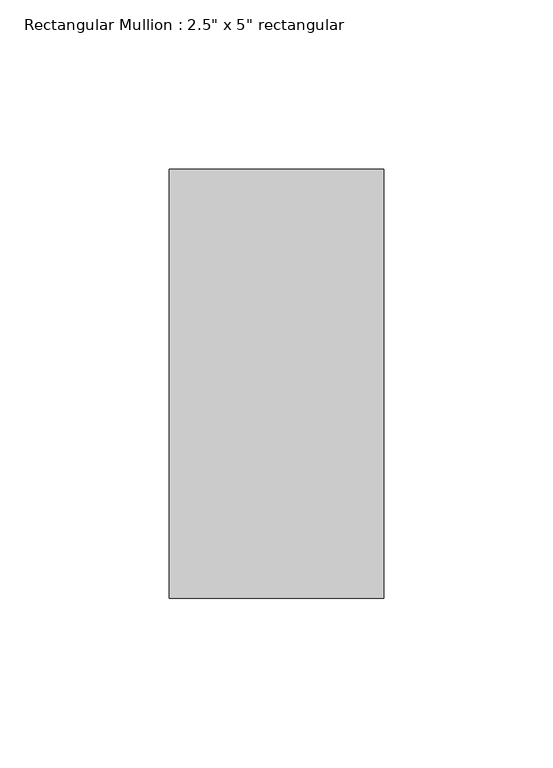
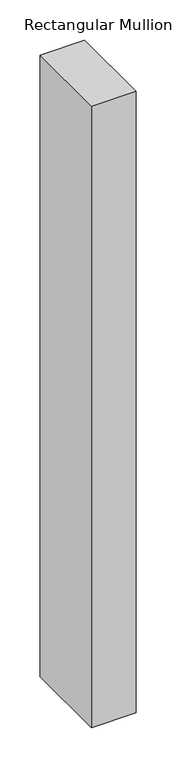
"""IFC4 building model written with IfcOpenShell, lengths in millimetres: member geometry."""

from ifc_helpers import new_model, si_unit, frame, origin, place, context, project, spatial, polyline, outline, extrude, source, transform, mapped, element, save


def member_ca079636(model_context):
    return source(origin(), model_context, "Body", "SweptSolid", [
        extrude(outline(polyline([(31.75, 63.5), (31.75, -63.5), (-31.75, -63.5), (-31.75, 63.5), (31.75, 63.5)])), frame((0.0, 0.0, -939.8), z_axis=(0.0, 0.0, 1.0), x_axis=(1.0, 0.0, 0.0)), (0.0, 0.0, 1.0), 939.8),
    ])


if __name__ == "__main__":
    model = new_model("IFC4")
    model_context = context("Model", 3, world=origin())
    ifc_project = project(units=[si_unit("LENGTHUNIT", "METRE", prefix="MILLI")], contexts=[model_context])
    site = spatial("IfcSite", under=ifc_project)
    building = spatial("IfcBuilding", under=site)
    placement = place(None, origin())
    member_shape = member_ca079636(model_context)
    element("IfcMember", 1, ObjectType="Rectangular Mullion : 2.5\" x 5\" rectangular", at=placement, inside=building, context=model_context, shape_type="MappedRepresentation", body=[
        mapped(member_shape, transform((0.0, 0.0, 0.0), x_axis=(1.0, 0.0, 0.0), y_axis=(0.0, 1.0, 0.0), z_axis=(0.0, 0.0, 1.0))),
    ])
    save(model, "model.ifc")

# Revit data of these elements
# Type "Rectangular Mullion : 2.5\" x 5\" rectangular"
#   built-in parameter 1007304 = 0.416667 (stored number, unit not read)
#   built-in parameter 1007301 = 0.104167 (stored number, unit not read)
#   built-in parameter 1007300 = 0.104167 (stored number, unit not read)
# Element 1 (IfcMember, "Rectangular Mullion : 2.5\" x 5\" rectangular")
#   Materials on its faces: "Aluminum"
# Materials
#   "Aluminum": class "Metal", colour RGB 247 247 247, transparency 0, Description = "Aluminum 6061", Cost = 0
